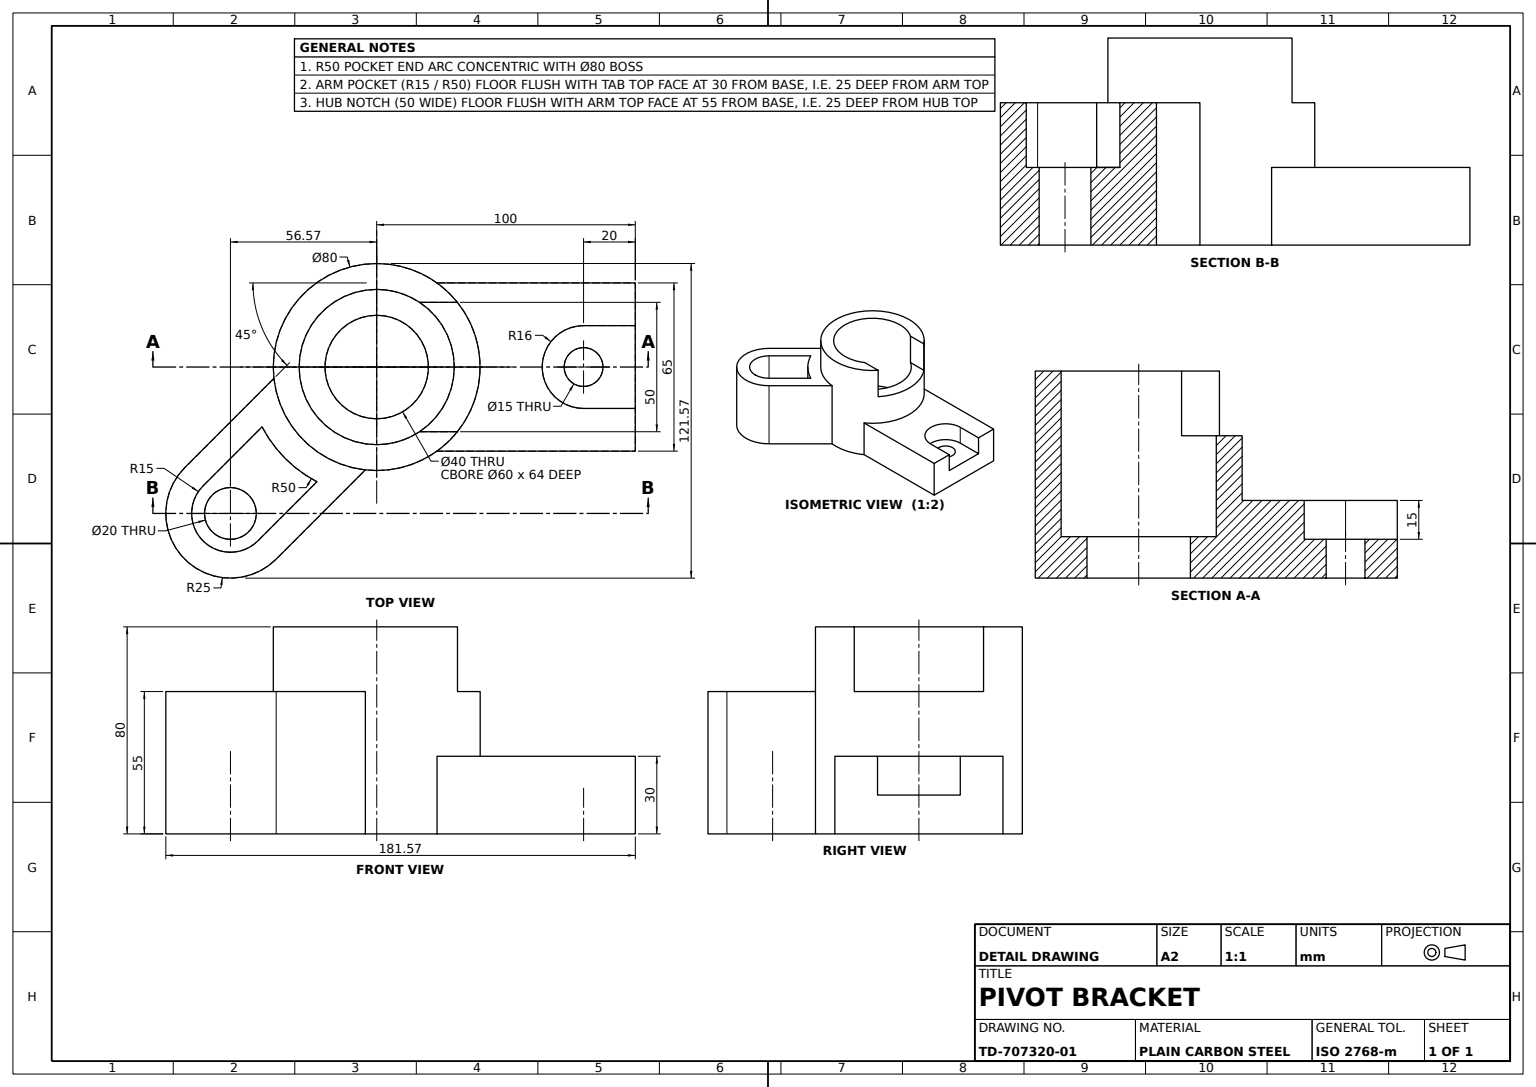
from build123d import *

# Parameters (mm, degrees)
HUB_PROFILE_SKETCH_R       = 40
HUB_CYLINDER_80_DEPTH      = 80
SIDE_TAB_DEPTH             = 55
ANGLED_ARM_45DEG_DEPTH     = 30
ARM_SLOT_POCKET_DEPTH      = 25
TAB_START                  = -25
TAB_SLOT_COUNTERBORE_DEPTH = 15
TAB_THROUGH_HOLE_REACH     = 142.28
HUB_START                  = 16
SKETCH1_3_R                = 30
HUB_BORE_60_DEPTH          = 64
HUB_WALL_NOTCH_REACH       = 153.834
HUB_NOTCH_SKETCH_R         = 10
HUB_NOTCH_SKETCH_R_2       = 7.5
HUB_NOTCH_SKETCH_R_3       = 20


with BuildPart() as part:
    # Hub Profile Sketch → Hub Cylinder _80 (new body)
    with BuildSketch(Plane(origin=(0, 0, 0), x_dir=(1, 0, 0), z_dir=(0, 1, 0))):
        with Locations(Location((0, 0, 0), (0, 0, 270))):
            Circle(HUB_PROFILE_SKETCH_R)
    extrude(amount=HUB_CYLINDER_80_DEPTH)

    # Arm and Tab Sketch → Side Tab (add)
    with BuildSketch(Plane(origin=(0, 0, 0), x_dir=(1, 0, 0), z_dir=(0, 1, 0))):
        with BuildLine():
            ThreePointArc((-39.757071695, -4.401732636), (-28.284271247, -28.284271247), (-4.401732636, -39.757071695))
            Line((-4.401732636, -39.757071695), (-38.890872965, -74.246212025))
            ThreePointArc((-38.890872965, -74.246212025), (-74.246212025, -74.246212025), (-74.246212025, -38.890872965))
            Line((-74.246212025, -38.890872965), (-39.757071695, -4.401732636))
        make_face()
    extrude(amount=SIDE_TAB_DEPTH)

    # Sketch3_3 → Angled Arm 45deg (add)
    with BuildSketch(Plane(origin=(0, 0, 0), x_dir=(1, 0, 0), z_dir=(0, 1, 0))):
        with BuildLine():
            ThreePointArc((23.318447633, -32.5), (40, 0), (23.318447633, 32.5))
            Line((23.318447633, 32.5), (100, 32.5))
            Line((100, 32.5), (100, -32.5))
            Line((100, -32.5), (23.318447633, -32.5))
        make_face()
    extrude(amount=ANGLED_ARM_45DEG_DEPTH)

    # Slot and Hole Sketch → Arm Slot Pocket (cut)
    with BuildSketch(Plane(origin=(0, 55, 0), x_dir=(1, 0, 0), z_dir=(0, 1, 0))):
        with BuildLine():
            Line((-44.333445626, -23.12024219), (-67.175144213, -45.961940777))
            ThreePointArc((-67.175144213, -45.961940777), (-67.175144213, -67.175144213), (-45.961940777, -67.175144213))
            Line((-45.961940777, -67.175144213), (-23.12024219, -44.333445626))
            ThreePointArc((-23.12024219, -44.333445626), (-35.355339059, -35.355339059), (-44.333445626, -23.12024219))
        make_face()
    extrude(amount=-ARM_SLOT_POCKET_DEPTH, mode=Mode.SUBTRACT)

    # Sketch4_3 → Tab Slot Counterbore (cut)
    with BuildSketch(Plane(origin=(0, 55, 0), x_dir=(1, 0, 0), z_dir=(0, 1, 0)).offset(TAB_START)):
        with BuildLine():
            Line((100, 16), (100, -16))
            Line((100, -16), (80, -16))
            ThreePointArc((80, -16), (64, 0), (80, 16))
            Line((80, 16), (100, 16))
        make_face()
    extrude(amount=-TAB_SLOT_COUNTERBORE_DEPTH, mode=Mode.SUBTRACT)

    # Sketch4_4 → Tab Through Hole (cut, up to next)
    with BuildSketch(Plane(origin=(0, 55, 0), x_dir=(1, 0, 0), z_dir=(0, 1, 0)), mode=Mode.PRIVATE) as tab_through_hole_sk1:
        with BuildLine():
            Line((16.583123952, 25), (31.224989992, 25))
            ThreePointArc((31.224989992, 25), (40, 0), (31.224989992, -25))
            Line((31.224989992, -25), (16.583123952, -25))
            ThreePointArc((16.583123952, -25), (30, 0), (16.583123952, 25))
        make_face()
    tab_through_hole_tool1 = extrude(tab_through_hole_sk1.sketch, amount=TAB_THROUGH_HOLE_REACH, mode=Mode.PRIVATE) & part.part
    add(tab_through_hole_tool1.solids().sort_by_distance((31.26913, 55, 0))[0], mode=Mode.SUBTRACT)

    # Sketch1_3 → Hub Bore _60 (cut)
    with BuildSketch(Plane(origin=(0, 0, 0), x_dir=(1, 0, 0), z_dir=(0, 1, 0)).offset(HUB_START)):
        with Locations(Location((0, 0, 0), (0, 0, 270))):
            Circle(SKETCH1_3_R)
    extrude(amount=HUB_BORE_60_DEPTH, mode=Mode.SUBTRACT)

    # Hub Notch Sketch → Hub Wall Notch (cut, up to next)
    with BuildSketch(Plane.XZ, mode=Mode.PRIVATE) as hub_wall_notch_sk1:
        with Locations(Location((-56.568542495, 56.568542495, 0), (0, 0, 270))):
            Circle(HUB_NOTCH_SKETCH_R)
    hub_wall_notch_tool1 = extrude(hub_wall_notch_sk1.sketch, amount=-HUB_WALL_NOTCH_REACH, mode=Mode.PRIVATE) & part.part
    # Hub Notch Sketch → Hub Wall Notch (cut, up to next)
    with BuildSketch(Plane.XZ, mode=Mode.PRIVATE) as hub_wall_notch_sk2:
        with Locations(Location((80, 0, 0), (0, 0, 270))):
            Circle(HUB_NOTCH_SKETCH_R_2)
    hub_wall_notch_tool2 = extrude(hub_wall_notch_sk2.sketch, amount=-HUB_WALL_NOTCH_REACH, mode=Mode.PRIVATE) & part.part
    # Hub Notch Sketch → Hub Wall Notch (cut, up to next)
    with BuildSketch(Plane.XZ, mode=Mode.PRIVATE) as hub_wall_notch_sk3:
        with Locations(Location((0, 0, 0), (0, 0, 270))):
            Circle(HUB_NOTCH_SKETCH_R_3)
    hub_wall_notch_tool3 = extrude(hub_wall_notch_sk3.sketch, amount=-HUB_WALL_NOTCH_REACH, mode=Mode.PRIVATE) & part.part
    add(hub_wall_notch_tool1.solids().sort_by_distance((-56.568542, 0, 56.568542))[0], mode=Mode.SUBTRACT)
    add(hub_wall_notch_tool2.solids().sort_by_distance((80, 0, 0))[0], mode=Mode.SUBTRACT)
    add(hub_wall_notch_tool3.solids().sort_by_distance((0, 0, 0))[0], mode=Mode.SUBTRACT)


solid = part.part
